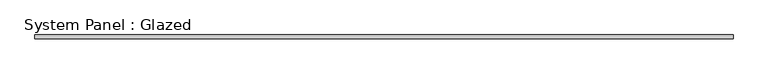
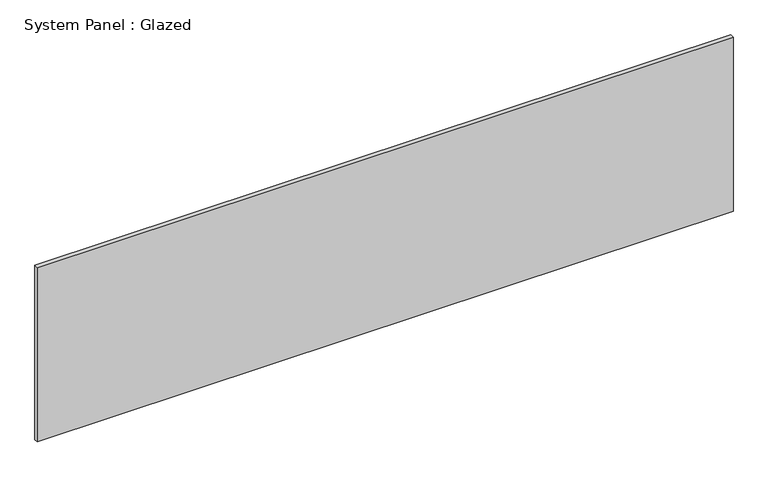
"""IFC4 building model written with IfcOpenShell, lengths in millimetres: plate geometry, System Panel : Glazed."""

from ifc_helpers import new_model, si_unit, origin, origin_with_axes, place, context, project, spatial, polyline, outline, extrude, source, transform, mapped, element, save


def system_panel_glazed_2c1c32f8(model_context):
    return source(origin(), model_context, "Body", "SweptSolid", [
        extrude(outline(polyline([(2303.6613302, 19.05), (-2303.6613302, 19.05), (-2303.6613302, 44.45), (2303.6613302, 44.45), (2303.6613302, 19.05)])), origin_with_axes(), (0.0, 0.0, 1.0), 1219.2),
    ])


if __name__ == "__main__":
    model = new_model("IFC4")
    model_context = context("Model", 3, world=origin())
    ifc_project = project(units=[si_unit("LENGTHUNIT", "METRE", prefix="MILLI")], contexts=[model_context])
    site = spatial("IfcSite", under=ifc_project)
    building = spatial("IfcBuilding", under=site)
    placement = place(None, origin())
    system_panel_glazed_shape = system_panel_glazed_2c1c32f8(model_context)
    element("IfcPlate", 1, ObjectType="System Panel : Glazed", at=placement, inside=building, context=model_context, shape_type="MappedRepresentation", body=[
        mapped(system_panel_glazed_shape, transform((0.0, 0.0, 0.0), x_axis=(1.0, 0.0, 0.0), y_axis=(0.0, 1.0, 0.0), z_axis=(0.0, 0.0, 1.0))),
    ])
    save(model, "model.ifc")

# Revit data of these elements
# Type "System Panel : Glazed"
#   Construction Type Id = "GSP4R"
#   Analytic Construction = "1/8 in Pilkington single glazing"
#   Visual Light Transmittance = 0.9
#   Solar Heat Gain Coefficient = 0.86
#   Heat Transfer Coefficient (U) = 1.18115 BTU/(h·ft²·°F)
# Element 1 (IfcPlate, "System Panel : Glazed")
#   Materials on its faces: "Glass"
# Materials
#   "Glass": class "Glass", colour RGB 0 128 192, transparency 0.75, Description = "Soda Lime Glass", Cost = 0
